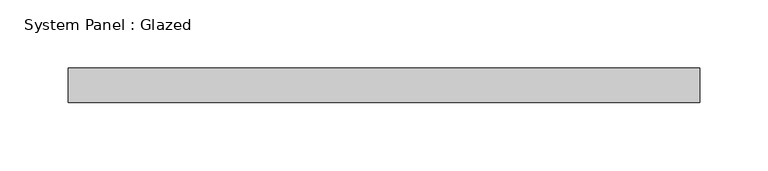
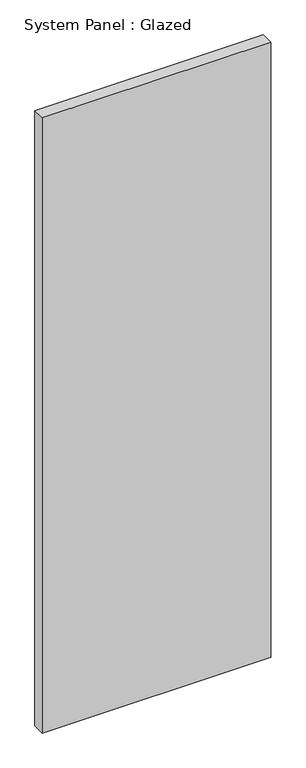
"""IFC4 building model written with IfcOpenShell, lengths in millimetres: plate geometry, System Panel : Glazed."""

from ifc_helpers import new_model, si_unit, origin, origin_with_axes, place, context, project, spatial, polyline, outline, extrude, source, transform, mapped, element, save


def system_panel_glazed_b47451c9(model_context):
    return source(origin(), model_context, "Body", "SweptSolid", [
        extrude(outline(polyline([(231.775, 19.05), (-231.775, 19.05), (-231.775, 44.45), (231.775, 44.45), (231.775, 19.05)])), origin_with_axes(), (0.0, 0.0, 1.0), 1319.9422272),
    ])


if __name__ == "__main__":
    model = new_model("IFC4")
    model_context = context("Model", 3, world=origin())
    ifc_project = project(units=[si_unit("LENGTHUNIT", "METRE", prefix="MILLI")], contexts=[model_context])
    site = spatial("IfcSite", under=ifc_project)
    building = spatial("IfcBuilding", under=site)
    placement = place(None, origin())
    system_panel_glazed_shape = system_panel_glazed_b47451c9(model_context)
    element("IfcPlate", 1, ObjectType="System Panel : Glazed", at=placement, inside=building, context=model_context, shape_type="MappedRepresentation", body=[
        mapped(system_panel_glazed_shape, transform((0.0, 0.0, 0.0), x_axis=(1.0, 0.0, 0.0), y_axis=(0.0, 1.0, 0.0), z_axis=(0.0, 0.0, 1.0))),
    ])
    save(model, "model.ifc")

# Revit data of these elements
# Type "System Panel : Glazed"
#   Construction Type Id = "GSP4R"
#   Analytic Construction = "1/8 in Pilkington single glazing"
#   Visual Light Transmittance = 0.9
#   Solar Heat Gain Coefficient = 0.86
#   Heat Transfer Coefficient (U) = 1.18115 BTU/(h·ft²·°F)
#   Define Thermal Properties by = 1
# Element 1 (IfcPlate, "System Panel : Glazed")
#   Materials on its faces: "Glass"
# Materials
#   "Glass": class "Glass", colour RGB 0 128 192, transparency 0.75, Description = "Soda Lime Glass", Cost = 0
